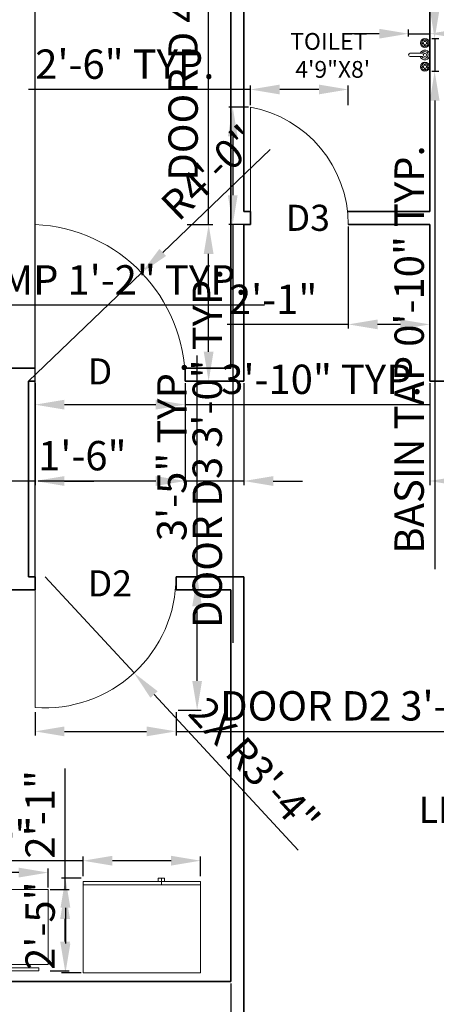
# Model space of a CAD drawing. Units: inches. Extents: x 2396 to 4051, y 1419 to 2191.
# Tile 3 of 7: x 2642 to 2770, y 1726 to 2028. Entities that reach past the tile are written whole.
import ezdxf

# ---------------------------------------------------------------- set-up
doc = ezdxf.new("R2010")
doc.units = ezdxf.units.IN
doc.layers.add('A-ANNO-TEXT', color=114, linetype='Continuous', lineweight=18, true_color=0x139b48)
for name, color, linetype, lineweight in [('A-AREA-IDEN', 6, 'Continuous', 18), ('A-DOOR', 4, 'Continuous', 18), ('A-EQPM', 8, 'Continuous', 18), ('A-FLOR-CASE', 9, 'Continuous', 18), ('A-FLOR-FIXT', 9, 'Continuous', 18), ('A-WALL', 7, 'Continuous', 35), ('S-ANNO-DIMS', 2, 'Continuous', 18)]:
    doc.layers.add(name, color=color, linetype=linetype, lineweight=lineweight)
doc.styles.get("Standard").update_dxf_attribs({"font": 'arial.ttf'})
doc.dimstyles.new('ISO-25', dxfattribs={"dimtxt": 9, "dimasz": 9, "dimexe": 1.25, "dimexo": 0.625, "dimgap": 2, "dimtad": 1, "dimdec": 1, "dimlunit": 4, "dimtxsty": 'Standard', "dimcen": 2.5, "dimadec": 0, "dimazin": 0, "dimtfac": 1, "dimtdec": 1, "dimtmove": 0, "dimatfit": 3, "dimfxl": 1, "dimarcsym": 0})

# ---------------------------------------------------------------- blocks, each defined once
blk = doc.blocks.new('Refrigerator-2 door - 36 in top')
for p, q in [((0, -26.999999), (36, -26.999999)), ((12, -26.999999), (12, -28.999999)), ((11, -27.999999), (11, -28.999999)), ((11, -28.999999), (13, -28.999999)), ((13, -28.999999), (13, -27.999999))]:
    blk.add_line(p, q)
blk.add_lwpolyline([(0, -27.999999), (0, 0), (36, 0), (36, -27.999999)], close=True)
blk = doc.blocks.new('Wall Cabinet - 18 x 12 in side')
for points in [[(-12, -18), (-12, 0), (0, 0), (0, -18)], [(-13, -16.5), (-13, -1.5), (-12.5, -1.5), (-12.5, -16.5)]]:
    blk.add_lwpolyline(points, close=True)
blk = doc.blocks.new('Faucet - Bathroom top')
for p, q in [((-4.107, 0.125), (-4.375, 0.125)), ((-3.75, 0.4788), (-3.75, 0.75)), ((-3.5, 0.482), (-3.5, 0.75)), ((-3.1461, 0.125), (-2.875, 0.125)), ((3.143, 0.125), (2.875, 0.125)), ((3.5, 0.4788), (3.5, 0.75)), ((3.75, 0.482), (3.75, 0.75)), ((4.1039, 0.125), (4.375, 0.125)), ((-4.1039, -0.125), (-4.375, -0.125)), ((-3.75, -0.4821), (-3.75, -0.75)), ((-3.5, -0.4789), (-3.5, -0.75)), ((-3.143, -0.125), (-2.875, -0.125)), ((-0.5, -0.8639), (-0.5, -4.5)), ((0.5, -4.5), (0.5, -0.8631)), ((3.1461, -0.125), (2.875, -0.125)), ((3.5, -0.4821), (3.5, -0.75)), ((3.75, -0.4789), (3.75, -0.75)), ((4.107, -0.125), (4.375, -0.125))]:
    blk.add_line(p, q)
for centre, radius in [((-3.625, 0), 1.375), ((-4.625, 0), 0.2795), ((-3.625, 0), 0.5), ((-3.625, 1), 0.2795), ((-2.625, 0), 0.2795), ((0, 0), 0.5), ((3.625, 0), 1.375), ((2.625, 0), 0.2795), ((3.625, 0), 0.5), ((3.625, 1), 0.2795), ((4.625, 0), 0.2795), ((-3.625, -1), 0.2795), ((3.625, -1), 0.2795)]:
    blk.add_circle(centre, radius)
for centre, radius, start, end in [((-3.625, 0), 1, 105.2407, 164.2093), ((-3.625, 0), 1, 16.44125, 74.07887), ((0, 0), 1.5, 289.6514, 250.3603), ((0, 0), 1, 300.3431, 239.7554), ((3.625, 0), 1, 106.12, 164.0884), ((3.625, 0), 1, 16.23422, 73.90469), ((-3.625, 0), 1, 196.2342, 253.9047), ((-3.625, 0), 1, 286.12, 344.0884), ((3.625, 0), 1, 196.4413, 254.0789), ((3.625, 0), 1, 285.2407, 344.2093), ((0, -4.5), 0.5, 180, 0)]:
    blk.add_arc(centre, radius, start, end)
blk = doc.blocks.new('DOOR-D-48IN')
blk.add_line((0, 0), (0, 48))
blk.add_arc((-2.04, 0), 48.04, 0, 87.5622)
blk = doc.blocks.new('DOOR-D3-36IN')
blk.add_line((30, 0), (30, 36))
blk.add_arc((36.6, 36), 36.6, 180, 259.6111)
blk = doc.blocks.new('DOOR-D2-40IN')
blk.add_line((0, 40.11), (0, 0.11))
blk.add_arc((3.08, 40.11), 40.12, 265.5948, 0)
blk = doc.blocks.new('*D40')
at = {"layer": 'Defpoints', "color": 0, "transparency": 16777216}
for p in [(2545.21, 1942.76), (2559.21, 1942.76), (2559.21, 1940.66)]:
    blk.add_point(p, dxfattribs=at)
at = {"layer": 'S-ANNO-DIMS', "color": 0, "lineweight": -2, "transparency": 16777216}
for p, q in [((2536.21, 1940.66), (2527.21, 1940.66)), ((2545.21, 1942.13), (2545.21, 1939.41)), ((2545.21, 1940.66), (2559.21, 1940.66)), ((2559.21, 1942.13), (2559.21, 1939.41)), ((2568.21, 1940.66), (2717.35, 1940.66))]:
    blk.add_line(p, q, dxfattribs=at)
at = {"layer": 'S-ANNO-DIMS', "color": 0, "transparency": 16777216}
for points in [[(2536.21, 1942.16), (2536.21, 1939.16), (2545.21, 1940.66)], [(2568.21, 1942.16), (2568.21, 1939.16), (2559.21, 1940.66)]]:
    blk.add_solid(points, dxfattribs=at)
at = {"layer": 'S-ANNO-DIMS', "color": 0, "transparency": 16777216, "insert": (2647.28, 1947.18), "char_height": 9, "attachment_point": 5}
blk.add_mtext('TABLE LAMP 1\'-2" TYP.', dxfattribs=at)
blk = doc.blocks.new('*D50')
at = {"layer": 'Defpoints', "color": 0, "transparency": 16777216}
for p in [(2767.98, 2022.3), (2767.98, 2012.3), (2769.48, 2012.3)]:
    blk.add_point(p, dxfattribs=at)
at = {"layer": 'S-ANNO-DIMS', "color": 0, "lineweight": -2, "transparency": 16777216}
for p, q in [((2769.48, 2031.3), (2769.48, 2040.3)), ((2768.61, 2022.3), (2770.73, 2022.3)), ((2769.48, 2022.3), (2769.48, 2012.3)), ((2768.61, 2012.3), (2770.73, 2012.3)), ((2769.48, 2003.3), (2769.48, 1859.68))]:
    blk.add_line(p, q, dxfattribs=at)
at = {"layer": 'S-ANNO-DIMS', "color": 0, "transparency": 16777216}
for points in [[(2767.98, 2031.3), (2770.98, 2031.3), (2769.48, 2022.3)], [(2767.98, 2003.3), (2770.98, 2003.3), (2769.48, 2012.3)]]:
    blk.add_solid(points, dxfattribs=at)
at = {"layer": 'S-ANNO-DIMS', "color": 0, "transparency": 16777216, "insert": (2762.83, 1926.99), "char_height": 9, "attachment_point": 5, "rotation": 90}
blk.add_mtext('BASIN TAP 0\'-10" TYP.', dxfattribs=at)
blk = doc.blocks.new('*D51')
at = {"layer": 'Defpoints', "color": 0, "transparency": 16777216}
for p in [(2761.48, 2022.3), (2767.98, 2023.8), (2767.98, 2022.3)]:
    blk.add_point(p, dxfattribs=at)
at = {"layer": 'S-ANNO-DIMS', "color": 0, "lineweight": -2, "transparency": 16777216}
for p, q in [((2761.48, 2022.93), (2761.48, 2025.05)), ((2767.98, 2022.93), (2767.98, 2025.05)), ((2752.48, 2023.8), (2743.48, 2023.8)), ((2761.48, 2023.8), (2767.98, 2023.8)), ((2776.98, 2023.8), (2865.81, 2023.8))]:
    blk.add_line(p, q, dxfattribs=at)
at = {"layer": 'S-ANNO-DIMS', "color": 0, "transparency": 16777216}
for points in [[(2752.48, 2025.3), (2752.48, 2022.3), (2761.48, 2023.8)], [(2776.98, 2025.3), (2776.98, 2022.3), (2767.98, 2023.8)]]:
    blk.add_solid(points, dxfattribs=at)
at = {"layer": 'S-ANNO-DIMS', "color": 0, "transparency": 16777216, "insert": (2825.9, 2030.45), "char_height": 9, "attachment_point": 5}
blk.add_mtext('0\'-6 1/2" TYP.', dxfattribs=at)
blk = doc.blocks.new('*D56')
at = {"layer": 'Defpoints', "color": 0, "transparency": 16777216}
for p in [(2692.98, 1965.3), (2700.18, 1965.3), (2692.98, 1917.3)]:
    blk.add_point(p, dxfattribs=at)
at = {"layer": 'S-ANNO-DIMS', "color": 0, "lineweight": -2, "transparency": 16777216}
for p, q in [((2700.18, 1965.3), (2700.18, 2086.5)), ((2693.61, 1965.3), (2701.43, 1965.3)), ((2700.18, 1926.3), (2700.18, 1956.3)), ((2693.61, 1917.3), (2701.43, 1917.3))]:
    blk.add_line(p, q, dxfattribs=at)
at = {"layer": 'S-ANNO-DIMS', "color": 0, "transparency": 16777216}
for points in [[(2698.68, 1956.3), (2701.68, 1956.3), (2700.18, 1965.3)], [(2698.68, 1926.3), (2701.68, 1926.3), (2700.18, 1917.3)]]:
    blk.add_solid(points, dxfattribs=at)
at = {"layer": 'S-ANNO-DIMS', "color": 0, "transparency": 16777216, "insert": (2693.53, 2030.4), "char_height": 9, "attachment_point": 5, "rotation": 90}
blk.add_mtext('DOOR D 4\'-0" TYP.', dxfattribs=at)
blk = doc.blocks.new('*D57')
at = {"layer": 'Defpoints', "color": 0, "transparency": 16777216}
for p in [(2646.98, 1917.3), (2692.98, 1917.3), (2692.98, 1910.1)]:
    blk.add_point(p, dxfattribs=at)
at = {"layer": 'S-ANNO-DIMS', "color": 0, "lineweight": -2, "transparency": 16777216}
for p, q in [((2646.98, 1916.68), (2646.98, 1908.85)), ((2692.98, 1916.68), (2692.98, 1908.85)), ((2655.98, 1910.1), (2683.98, 1910.1)), ((2692.98, 1910.1), (2767.83, 1910.1))]:
    blk.add_line(p, q, dxfattribs=at)
at = {"layer": 'S-ANNO-DIMS', "color": 0, "transparency": 16777216}
for points in [[(2655.98, 1911.6), (2655.98, 1908.6), (2646.98, 1910.1)], [(2683.98, 1911.6), (2683.98, 1908.6), (2692.98, 1910.1)]]:
    blk.add_solid(points, dxfattribs=at)
at = {"layer": 'S-ANNO-DIMS', "color": 0, "transparency": 16777216, "insert": (2734.91, 1916.7), "char_height": 9, "attachment_point": 5}
blk.add_mtext('3\'-10" TYP.', dxfattribs=at)
blk = doc.blocks.new('*D58')
at = {"layer": 'Defpoints', "color": 0, "transparency": 16777216}
for p in [(2712.98, 2001.3), (2707.58, 1965.3), (2712.98, 1965.3)]:
    blk.add_point(p, dxfattribs=at)
at = {"layer": 'S-ANNO-DIMS', "color": 0, "lineweight": -2, "transparency": 16777216}
for p, q in [((2712.36, 2001.3), (2706.33, 2001.3)), ((2707.58, 1992.3), (2707.58, 1974.3)), ((2712.36, 1965.3), (2706.33, 1965.3)), ((2707.58, 1965.3), (2707.58, 1837.11))]:
    blk.add_line(p, q, dxfattribs=at)
at = {"layer": 'S-ANNO-DIMS', "color": 0, "transparency": 16777216}
for points in [[(2706.08, 1992.3), (2709.08, 1992.3), (2707.58, 2001.3)], [(2706.08, 1974.3), (2709.08, 1974.3), (2707.58, 1965.3)]]:
    blk.add_solid(points, dxfattribs=at)
at = {"layer": 'S-ANNO-DIMS', "color": 0, "transparency": 16777216, "insert": (2700.92, 1896.71), "char_height": 9, "attachment_point": 5, "rotation": 90}
blk.add_mtext('DOOR D3 3\'-0" TYP.', dxfattribs=at)
blk = doc.blocks.new('*D59')
at = {"layer": 'Defpoints', "color": 0, "transparency": 16777216}
for p in [(2712.98, 2006.7), (2712.98, 2001.3), (2742.98, 2001.3)]:
    blk.add_point(p, dxfattribs=at)
at = {"layer": 'S-ANNO-DIMS', "color": 0, "lineweight": -2, "transparency": 16777216}
for p, q in [((2712.98, 2001.93), (2712.98, 2007.95)), ((2742.98, 2001.93), (2742.98, 2007.95)), ((2712.98, 2006.7), (2644.97, 2006.7)), ((2733.98, 2006.7), (2721.98, 2006.7))]:
    blk.add_line(p, q, dxfattribs=at)
at = {"layer": 'S-ANNO-DIMS', "color": 0, "transparency": 16777216}
for points in [[(2721.98, 2008.2), (2721.98, 2005.2), (2712.98, 2006.7)], [(2733.98, 2008.2), (2733.98, 2005.2), (2742.98, 2006.7)]]:
    blk.add_solid(points, dxfattribs=at)
at = {"layer": 'S-ANNO-DIMS', "color": 0, "transparency": 16777216, "insert": (2674.48, 2013.3), "char_height": 9, "attachment_point": 5}
blk.add_mtext('2\'-6" TYP.', dxfattribs=at)
blk = doc.blocks.new('*D60')
at = {"layer": 'Defpoints', "color": 0, "transparency": 16777216}
for p in [(2646.98, 1816.44), (2690.18, 1816.44), (2690.18, 1809.96)]:
    blk.add_point(p, dxfattribs=at)
at = {"layer": 'S-ANNO-DIMS', "color": 0, "lineweight": -2, "transparency": 16777216}
for p, q in [((2646.98, 1815.82), (2646.98, 1808.71)), ((2690.18, 1815.82), (2690.18, 1808.71)), ((2655.98, 1809.96), (2681.18, 1809.96)), ((2690.18, 1809.96), (2818.37, 1809.96))]:
    blk.add_line(p, q, dxfattribs=at)
at = {"layer": 'S-ANNO-DIMS', "color": 0, "transparency": 16777216}
for points in [[(2655.98, 1811.46), (2655.98, 1808.46), (2646.98, 1809.96)], [(2681.18, 1811.46), (2681.18, 1808.46), (2690.18, 1809.96)]]:
    blk.add_solid(points, dxfattribs=at)
at = {"layer": 'S-ANNO-DIMS', "color": 0, "transparency": 16777216, "insert": (2758.78, 1816.62), "char_height": 9, "attachment_point": 5}
blk.add_mtext('DOOR D2 3\'-7" TYP.', dxfattribs=at)
blk = doc.blocks.new('*D61')
at = {"layer": 'Defpoints', "color": 0, "transparency": 16777216}
for p in [(2690.18, 1857.3), (2696.66, 1857.3), (2690.18, 1816.44)]:
    blk.add_point(p, dxfattribs=at)
at = {"layer": 'S-ANNO-DIMS', "color": 0, "lineweight": -2, "transparency": 16777216}
for p, q in [((2696.66, 1857.3), (2696.66, 1925.15)), ((2690.81, 1857.3), (2697.91, 1857.3)), ((2696.66, 1825.44), (2696.66, 1848.3)), ((2690.81, 1816.44), (2697.91, 1816.44))]:
    blk.add_line(p, q, dxfattribs=at)
at = {"layer": 'S-ANNO-DIMS', "color": 0, "transparency": 16777216}
for points in [[(2695.16, 1848.3), (2698.16, 1848.3), (2696.66, 1857.3)], [(2695.16, 1825.44), (2698.16, 1825.44), (2696.66, 1816.44)]]:
    blk.add_solid(points, dxfattribs=at)
at = {"layer": 'S-ANNO-DIMS', "color": 0, "transparency": 16777216, "insert": (2690.07, 1895.73), "char_height": 9, "attachment_point": 5, "rotation": 90}
blk.add_mtext('3\'-5" TYP.', dxfattribs=at)
blk = doc.blocks.new('*D66')
at = {"layer": 'Defpoints', "color": 0, "transparency": 16777216}
for p in [(2661.68, 1770.32), (2661.68, 1764.92), (2697.68, 1764.92)]:
    blk.add_point(p, dxfattribs=at)
at = {"layer": 'S-ANNO-DIMS', "color": 0, "lineweight": -2, "transparency": 16777216}
for p, q in [((2661.68, 1765.55), (2661.68, 1771.57)), ((2697.68, 1765.55), (2697.68, 1771.57)), ((2661.68, 1770.32), (2521.84, 1770.32)), ((2688.68, 1770.32), (2670.68, 1770.32))]:
    blk.add_line(p, q, dxfattribs=at)
at = {"layer": 'S-ANNO-DIMS', "color": 0, "transparency": 16777216}
for points in [[(2670.68, 1771.82), (2670.68, 1768.82), (2661.68, 1770.32)], [(2688.68, 1771.82), (2688.68, 1768.82), (2697.68, 1770.32)]]:
    blk.add_solid(points, dxfattribs=at)
at = {"layer": 'S-ANNO-DIMS', "color": 0, "transparency": 16777216, "insert": (2587.26, 1776.98), "char_height": 9, "attachment_point": 5}
blk.add_mtext('REFRIGERATOR 3\'-0"', dxfattribs=at)
blk = doc.blocks.new('*D67')
at = {"layer": 'Defpoints', "color": 0, "transparency": 16777216}
for p in [(2661.68, 1764.92), (2656.28, 1735.92), (2661.68, 1735.92)]:
    blk.add_point(p, dxfattribs=at)
at = {"layer": 'S-ANNO-DIMS', "color": 0, "lineweight": -2, "transparency": 16777216}
for p, q in [((2661.06, 1764.92), (2655.03, 1764.92)), ((2656.28, 1755.92), (2656.28, 1744.92)), ((2661.06, 1735.92), (2655.03, 1735.92))]:
    blk.add_line(p, q, dxfattribs=at)
at = {"layer": 'S-ANNO-DIMS', "color": 0, "transparency": 16777216}
for points in [[(2654.78, 1755.92), (2657.78, 1755.92), (2656.28, 1764.92)], [(2654.78, 1744.92), (2657.78, 1744.92), (2656.28, 1735.92)]]:
    blk.add_solid(points, dxfattribs=at)
at = {"layer": 'S-ANNO-DIMS', "color": 0, "transparency": 16777216, "insert": (2649.69, 1750.42), "char_height": 9, "attachment_point": 5, "rotation": 90}
blk.add_mtext('2\'-5"', dxfattribs=at)
blk = doc.blocks.new('*D68')
at = {"layer": 'Defpoints', "color": 0, "transparency": 16777216}
for p in [(2616.45, 1766.68), (2616.45, 1761.5), (2650.99, 1761.5)]:
    blk.add_point(p, dxfattribs=at)
at = {"layer": 'S-ANNO-DIMS', "color": 0, "lineweight": -2, "transparency": 16777216}
for p, q in [((2616.45, 1766.68), (2493.68, 1766.68)), ((2616.45, 1762.12), (2616.45, 1767.93)), ((2641.99, 1766.68), (2625.45, 1766.68)), ((2650.99, 1762.12), (2650.99, 1767.93))]:
    blk.add_line(p, q, dxfattribs=at)
at = {"layer": 'S-ANNO-DIMS', "color": 0, "transparency": 16777216}
for points in [[(2625.45, 1768.18), (2625.45, 1765.18), (2616.45, 1766.68)], [(2641.99, 1768.18), (2641.99, 1765.18), (2650.99, 1766.68)]]:
    blk.add_solid(points, dxfattribs=at)
at = {"layer": 'S-ANNO-DIMS', "color": 0, "transparency": 16777216, "insert": (2550.56, 1773.33), "char_height": 9, "attachment_point": 5}
blk.add_mtext('CABINET 2\'-10 1/2"', dxfattribs=at)
blk = doc.blocks.new('*D69')
at = {"layer": 'Defpoints', "color": 0, "transparency": 16777216}
for p in [(2650.99, 1761.5), (2656.17, 1761.5), (2650.99, 1736.54)]:
    blk.add_point(p, dxfattribs=at)
at = {"layer": 'S-ANNO-DIMS', "color": 0, "lineweight": -2, "transparency": 16777216}
for p, q in [((2656.17, 1761.5), (2656.17, 1798.57)), ((2651.62, 1761.5), (2657.42, 1761.5)), ((2656.17, 1745.54), (2656.17, 1752.5)), ((2651.62, 1736.54), (2657.42, 1736.54))]:
    blk.add_line(p, q, dxfattribs=at)
at = {"layer": 'S-ANNO-DIMS', "color": 0, "transparency": 16777216}
for points in [[(2654.67, 1752.5), (2657.67, 1752.5), (2656.17, 1761.5)], [(2654.67, 1745.54), (2657.67, 1745.54), (2656.17, 1736.54)]]:
    blk.add_solid(points, dxfattribs=at)
at = {"layer": 'S-ANNO-DIMS', "color": 0, "transparency": 16777216, "insert": (2649.66, 1784.53), "char_height": 9, "attachment_point": 5, "rotation": 90}
blk.add_mtext('2\'-1"', dxfattribs=at)
blk = doc.blocks.new('*D77')
at = {"layer": 'Defpoints', "color": 0, "transparency": 16777216}
for p in [(2529.98, 2074.3), (2499.38, 1534.3), (2774.98, 1534.3)]:
    blk.add_point(p, dxfattribs=at)
at = {"layer": 'S-ANNO-DIMS', "color": 0, "lineweight": -2, "transparency": 16777216}
for p, q in [((2529.36, 2074.3), (2498.13, 2074.3)), ((2499.38, 2065.3), (2499.38, 1543.3)), ((2774.36, 1534.3), (2498.13, 1534.3))]:
    blk.add_line(p, q, dxfattribs=at)
at = {"layer": 'S-ANNO-DIMS', "color": 0, "transparency": 16777216}
for points in [[(2497.88, 2065.3), (2500.88, 2065.3), (2499.38, 2074.3)], [(2497.88, 1543.3), (2500.88, 1543.3), (2499.38, 1534.3)]]:
    blk.add_solid(points, dxfattribs=at)
at = {"layer": 'S-ANNO-DIMS', "color": 0, "transparency": 16777216, "insert": (2492.79, 1804.3), "char_height": 9, "attachment_point": 5, "rotation": 90}
blk.add_mtext('45\'-0"', dxfattribs=at)
blk = doc.blocks.new('*D78')
at = {"layer": 'Defpoints', "color": 0, "transparency": 16777216}
for p in [(2538.98, 1733.3), (2706.98, 1733.3), (2706.98, 1503.7)]:
    blk.add_point(p, dxfattribs=at)
at = {"layer": 'S-ANNO-DIMS', "color": 0, "lineweight": -2, "transparency": 16777216}
for p, q in [((2538.98, 1732.68), (2538.98, 1502.45)), ((2706.98, 1732.68), (2706.98, 1502.45)), ((2547.98, 1503.7), (2697.98, 1503.7))]:
    blk.add_line(p, q, dxfattribs=at)
at = {"layer": 'S-ANNO-DIMS', "color": 0, "transparency": 16777216}
for points in [[(2547.98, 1505.2), (2547.98, 1502.2), (2538.98, 1503.7)], [(2697.98, 1505.2), (2697.98, 1502.2), (2706.98, 1503.7)]]:
    blk.add_solid(points, dxfattribs=at)
at = {"layer": 'S-ANNO-DIMS', "color": 0, "transparency": 16777216, "insert": (2622.98, 1510.3), "char_height": 9, "attachment_point": 5}
blk.add_mtext('14\'-0"', dxfattribs=at)
blk = doc.blocks.new('*D94')
at = {"layer": 'Defpoints', "color": 0, "transparency": 16777216}
for p in [(2767.98, 1917.3), (2846.98, 1917.3), (2767.98, 1886.7)]:
    blk.add_point(p, dxfattribs=at)
at = {"layer": 'S-ANNO-DIMS', "color": 0, "lineweight": -2, "transparency": 16777216}
for p, q in [((2767.98, 1916.68), (2767.98, 1885.45)), ((2846.98, 1916.68), (2846.98, 1885.45)), ((2837.98, 1886.7), (2776.98, 1886.7))]:
    blk.add_line(p, q, dxfattribs=at)
at = {"layer": 'S-ANNO-DIMS', "color": 0, "transparency": 16777216}
for points in [[(2776.98, 1888.2), (2776.98, 1885.2), (2767.98, 1886.7)], [(2837.98, 1888.2), (2837.98, 1885.2), (2846.98, 1886.7)]]:
    blk.add_solid(points, dxfattribs=at)
at = {"layer": 'S-ANNO-DIMS', "color": 0, "transparency": 16777216, "insert": (2807.48, 1893.3), "char_height": 9, "attachment_point": 5}
blk.add_mtext('6\'-7"', dxfattribs=at)
blk = doc.blocks.new('*D95')
at = {"layer": 'Defpoints', "color": 0, "transparency": 16777216}
for p in [(2646.98, 2154.77), (2538.98, 1853.3), (2646.98, 1853.3)]:
    blk.add_point(p, dxfattribs=at)
at = {"layer": 'S-ANNO-DIMS', "color": 0, "lineweight": -2, "transparency": 16777216}
for p, q in [((2538.98, 1853.93), (2538.98, 2156.02)), ((2547.98, 2154.77), (2637.98, 2154.77)), ((2646.98, 1853.93), (2646.98, 2156.02))]:
    blk.add_line(p, q, dxfattribs=at)
at = {"layer": 'S-ANNO-DIMS', "color": 0, "transparency": 16777216}
for points in [[(2547.98, 2156.27), (2547.98, 2153.27), (2538.98, 2154.77)], [(2637.98, 2156.27), (2637.98, 2153.27), (2646.98, 2154.77)]]:
    blk.add_solid(points, dxfattribs=at)
at = {"layer": 'S-ANNO-DIMS', "color": 0, "transparency": 16777216, "insert": (2592.98, 2161.37), "char_height": 9, "attachment_point": 5}
blk.add_mtext('9\'-0"', dxfattribs=at)
blk = doc.blocks.new('*D97')
at = {"layer": 'Defpoints', "color": 0, "transparency": 16777216}
for p in [(2692.98, 1917.3), (2710.98, 1917.3), (2692.98, 1886.7)]:
    blk.add_point(p, dxfattribs=at)
at = {"layer": 'S-ANNO-DIMS', "color": 0, "lineweight": -2, "transparency": 16777216}
for p, q in [((2692.98, 1916.68), (2692.98, 1885.45)), ((2710.98, 1916.68), (2710.98, 1885.45)), ((2683.98, 1886.7), (2647.91, 1886.7)), ((2710.98, 1886.7), (2692.98, 1886.7)), ((2719.98, 1886.7), (2728.98, 1886.7))]:
    blk.add_line(p, q, dxfattribs=at)
at = {"layer": 'S-ANNO-DIMS', "color": 0, "transparency": 16777216}
for points in [[(2683.98, 1888.2), (2683.98, 1885.2), (2692.98, 1886.7)], [(2719.98, 1888.2), (2719.98, 1885.2), (2710.98, 1886.7)]]:
    blk.add_solid(points, dxfattribs=at)
at = {"layer": 'S-ANNO-DIMS', "color": 0, "transparency": 16777216, "insert": (2661.45, 1893.3), "char_height": 9, "attachment_point": 5}
blk.add_mtext('1\'-6"', dxfattribs=at)
blk = doc.blocks.new('*D98')
at = {"layer": 'Defpoints', "color": 0, "transparency": 16777216}
for p in [(2629.98, 1917.3), (2646.98, 1917.3), (2629.98, 1886.7)]:
    blk.add_point(p, dxfattribs=at)
at = {"layer": 'S-ANNO-DIMS', "color": 0, "lineweight": -2, "transparency": 16777216}
for p, q in [((2629.98, 1916.68), (2629.98, 1885.45)), ((2646.98, 1916.68), (2646.98, 1885.45)), ((2620.98, 1886.7), (2584.91, 1886.7)), ((2646.98, 1886.7), (2629.98, 1886.7)), ((2655.98, 1886.7), (2664.98, 1886.7))]:
    blk.add_line(p, q, dxfattribs=at)
at = {"layer": 'S-ANNO-DIMS', "color": 0, "transparency": 16777216}
for points in [[(2620.98, 1888.2), (2620.98, 1885.2), (2629.98, 1886.7)], [(2655.98, 1888.2), (2655.98, 1885.2), (2646.98, 1886.7)]]:
    blk.add_solid(points, dxfattribs=at)
at = {"layer": 'S-ANNO-DIMS', "color": 0, "transparency": 16777216, "insert": (2598.45, 1893.3), "char_height": 9, "attachment_point": 5}
blk.add_mtext('1\'-5"', dxfattribs=at)
blk = doc.blocks.new('*D99')
at = {"layer": 'Defpoints', "color": 0, "transparency": 16777216}
for p in [(2742.98, 1965.3), (2767.98, 1965.3), (2742.98, 1934.7)]:
    blk.add_point(p, dxfattribs=at)
at = {"layer": 'S-ANNO-DIMS', "color": 0, "lineweight": -2, "transparency": 16777216}
for p, q in [((2742.98, 1964.68), (2742.98, 1933.45)), ((2767.98, 1964.68), (2767.98, 1933.45)), ((2742.98, 1934.7), (2705.91, 1934.7)), ((2758.98, 1934.7), (2751.98, 1934.7))]:
    blk.add_line(p, q, dxfattribs=at)
at = {"layer": 'S-ANNO-DIMS', "color": 0, "transparency": 16777216}
for points in [[(2751.98, 1936.2), (2751.98, 1933.2), (2742.98, 1934.7)], [(2758.98, 1936.2), (2758.98, 1933.2), (2767.98, 1934.7)]]:
    blk.add_solid(points, dxfattribs=at)
at = {"layer": 'S-ANNO-DIMS', "color": 0, "transparency": 16777216, "insert": (2719.95, 1941.22), "char_height": 9, "attachment_point": 5}
blk.add_mtext('2\'-1"', dxfattribs=at)
blk = doc.blocks.new('*D113')
at = {"layer": 'Defpoints', "color": 0, "transparency": 16777216}
for p in [(2679.63, 1950.54), (2644.94, 1917.3)]:
    blk.add_point(p, dxfattribs=at)
at = {"layer": 'S-ANNO-DIMS', "color": 0, "lineweight": -2, "transparency": 16777216}
for p, q in [((2719, 1988.28), (2686.13, 1956.77)), ((2644.94, 1917.3), (2679.63, 1950.54))]:
    blk.add_line(p, q, dxfattribs=at)
at = {"layer": 'S-ANNO-DIMS', "color": 0, "transparency": 16777216}
blk.add_solid([(2685.09, 1957.85), (2687.16, 1955.69), (2679.63, 1950.54)], dxfattribs=at)
at = {"layer": 'S-ANNO-DIMS', "color": 0, "transparency": 16777216, "insert": (2701.25, 1980.4), "char_height": 9, "attachment_point": 5, "rotation": 43.7812}
blk.add_mtext('R4\'-0"', dxfattribs=at)
blk = doc.blocks.new('*D114')
at = {"layer": 'Defpoints', "color": 0, "transparency": 16777216}
for p in [(2650.07, 1857.3), (2677.32, 1827.86)]:
    blk.add_point(p, dxfattribs=at)
at = {"layer": 'S-ANNO-DIMS', "color": 0, "lineweight": -2, "transparency": 16777216}
for p, q in [((2650.07, 1857.3), (2677.32, 1827.86)), ((2727.62, 1773.54), (2683.44, 1821.26))]:
    blk.add_line(p, q, dxfattribs=at)
at = {"layer": 'S-ANNO-DIMS', "color": 0, "transparency": 16777216}
blk.add_solid([(2684.54, 1822.28), (2682.34, 1820.24), (2677.32, 1827.86)], dxfattribs=at)
at = {"layer": 'S-ANNO-DIMS', "color": 0, "transparency": 16777216, "insert": (2713.43, 1798.58), "char_height": 9, "attachment_point": 5, "rotation": 312.7969}
blk.add_mtext('2X R3\'-4"', dxfattribs=at)

msp = doc.modelspace()

# ---------------------------------------------------------------- linework, layer by layer
at = {"layer": 'A-WALL'}
for p, q in [((2706.98, 2065.3), (2706.98, 1921.3)), ((2710.98, 2065.3), (2710.98, 1969.3)), ((2767.98, 2065.3), (2767.98, 1969.3)), ((2710.98, 1969.3), (2712.98, 1969.3)), ((2712.98, 1969.3), (2712.98, 1965.3)), ((2742.76, 1969.3), (2767.98, 1969.3)), ((2710.98, 1965.3), (2712.98, 1965.3)), ((2710.98, 1965.3), (2710.98, 1917.3)), ((2742.98, 1965.3), (2767.98, 1965.3)), ((2767.98, 1965.3), (2767.98, 1917.3)), ((2646.98, 1921.3), (2629.98, 1921.3)), ((2706.98, 1921.3), (2692.98, 1921.3)), ((2692.98, 1917.3), (2692.98, 1921.3)), ((2644.98, 1857.3), (2644.98, 1917.3)), ((2646.98, 1917.3), (2644.98, 1917.3)), ((2710.98, 1917.3), (2692.98, 1917.3)), ((2846.98, 1917.3), (2767.98, 1917.3)), ((2646.98, 1857.3), (2644.98, 1857.3)), ((2646.98, 1853.3), (2646.98, 1857.3)), ((2710.98, 1857.3), (2690.18, 1857.3)), ((2690.18, 1853.3), (2690.18, 1857.3)), ((2710.98, 1857.3), (2710.98, 1632.3)), ((2644.98, 1853.3), (2538.98, 1853.3)), ((2646.98, 1853.3), (2644.98, 1853.3)), ((2706.98, 1853.3), (2690.18, 1853.3)), ((2706.98, 1853.3), (2706.98, 1733.3)), ((2706.98, 1733.3), (2538.98, 1733.3))]:
    msp.add_line(p, q, dxfattribs=at)

# ---------------------------------------------------------------- block references
at = {"layer": 'A-DOOR', "rotation": 180}
msp.add_blockref('DOOR-D3-36IN', (2742.98, 2001.3), dxfattribs=at)
at = {"layer": 'A-DOOR'}
for name, p in [('DOOR-D-48IN', (2646.98, 1917.3)), ('DOOR-D2-40IN', (2646.98, 1817.19))]:
    msp.add_blockref(name, p, dxfattribs=at)
at = {"layer": 'A-EQPM', "rotation": 180}
msp.add_blockref('Refrigerator-2 door - 36 in top', (2697.68, 1735.92), dxfattribs=at)
at = {"layer": 'A-FLOR-CASE', "xscale": 1.91927912988188, "yscale": 1.91927912988188, "zscale": 1.91927912988188, "rotation": 90}
msp.add_blockref('Wall Cabinet - 18 x 12 in side', (2616.45, 1761.5), dxfattribs=at)
at = {"layer": 'A-FLOR-FIXT', "rotation": 270}
msp.add_blockref('Faucet - Bathroom top', (2766.48, 2017.3), dxfattribs=at)

# ---------------------------------------------------------------- texts
at = {"layer": 'A-ANNO-TEXT', "char_height": 8, "attachment_point": 1}
for s, insert in [('{D3}', (2723.8, 1971.37)), ('{D}', (2663.12, 1924.28)), ('{D2}', (2663.12, 1859.32))]:
    msp.add_mtext_dynamic_manual_height_columns(s, width=139.3028, gutter_width=12.5, heights=[0], dxfattribs=dict(at, insert=insert))
at = {"layer": 'A-AREA-IDEN', "attachment_point": 1}
for s, width, gutter_width, insert, char_height in [('   TOILET\\P    4\'9"X8\'', 89.5376, 8.03, (2720.48, 2024.01), 5.142), ("   LIVING ROOM\\P        15'X23'", 139.3028, 12.5, (2757.3, 1789.91), 8)]:
    msp.add_mtext_dynamic_manual_height_columns(s, width=width, gutter_width=gutter_width, heights=[0], dxfattribs=dict(at, insert=insert, char_height=char_height))

# ---------------------------------------------------------------- dimensions: what is measured, and where the dimension line sits
at = {"layer": 'S-ANNO-DIMS'}
for base, p1, p2, picture, middle in [((2646.98, 2154.77), (2538.98, 1853.3), (2646.98, 1853.3), '*D95', (2592.98, 2161.37)), ((2706.98, 1503.7), (2538.98, 1733.3), (2706.98, 1733.3), '*D78', (2622.98, 1510.3))]:
    dim = msp.add_linear_dim(base=base, p1=p1, p2=p2, dimstyle='ISO-25', override={"dimdec": 1, "dimlfac": 1, "dimrnd": 0, "dimzin": 1, "dimdsep": 46, "dimlunit": 4, "dimfrac": 2}, dxfattribs=at)
    dim.commit()
    dim.dimension.update_dxf_attribs({"geometry": picture, "text_midpoint": middle})
for base, p1, p2, angle, text, picture, middle in [((2700.18, 1965.3), (2692.98, 1917.3), (2692.98, 1965.3), 90, 'DOOR D <> TYP.', '*D56', (2693.53, 2030.4)), ((2769.48, 2012.3), (2767.98, 2022.3), (2767.98, 2012.3), 270, 'BASIN TAP <> TYP.', '*D50', (2762.83, 1926.99)), ((2712.98, 2006.7), (2742.98, 2001.3), (2712.98, 2001.3), 180, '<> TYP.', '*D59', (2674.48, 2013.3)), ((2707.58, 1965.3), (2712.98, 2001.3), (2712.98, 1965.3), 270, 'DOOR D3 <> TYP.', '*D58', (2700.92, 1896.71)), ((2696.66, 1857.3), (2690.18, 1816.44), (2690.18, 1857.3), 90, '<> TYP.', '*D61', (2690.07, 1895.73)), ((2616.45, 1766.68), (2650.99, 1761.5), (2616.45, 1761.5), 180, 'CABINET <>', '*D68', (2550.56, 1773.33)), ((2661.68, 1770.32), (2697.68, 1764.92), (2661.68, 1764.92), 180, 'REFRIGERATOR <>', '*D66', (2587.26, 1776.98))]:
    dim = msp.add_linear_dim(base=base, p1=p1, p2=p2, angle=angle, text=text, dimstyle='ISO-25', override={"dimdec": 1, "dimlfac": 1, "dimrnd": 0, "dimzin": 1, "dimdsep": 46, "dimlunit": 4, "dimfrac": 2}, dxfattribs=at)
    dim.commit()
    dim.dimension.update_dxf_attribs({"geometry": picture, "text_midpoint": middle})
for base, p1, p2, angle, picture, middle in [((2499.38, 1534.3), (2529.98, 2074.3), (2774.98, 1534.3), 90, '*D77', (2492.79, 1804.3)), ((2742.98, 1934.7), (2767.98, 1965.3), (2742.98, 1965.3), 180, '*D99', (2719.95, 1941.22)), ((2629.98, 1886.7), (2646.98, 1917.3), (2629.98, 1917.3), 180, '*D98', (2598.45, 1893.3)), ((2692.98, 1886.7), (2710.98, 1917.3), (2692.98, 1917.3), 180, '*D97', (2661.45, 1893.3)), ((2767.98, 1886.7), (2846.98, 1917.3), (2767.98, 1917.3), 180, '*D94', (2807.48, 1893.3)), ((2656.17, 1761.5), (2650.99, 1736.54), (2650.99, 1761.5), 90, '*D69', (2649.66, 1784.53)), ((2656.28, 1735.92), (2661.68, 1764.92), (2661.68, 1735.92), 270, '*D67', (2649.69, 1750.42))]:
    dim = msp.add_linear_dim(base=base, p1=p1, p2=p2, angle=angle, dimstyle='ISO-25', override={"dimdec": 1, "dimlfac": 1, "dimrnd": 0, "dimzin": 1, "dimdsep": 46, "dimlunit": 4, "dimfrac": 2}, dxfattribs=at)
    dim.commit()
    dim.dimension.update_dxf_attribs({"geometry": picture, "text_midpoint": middle})
for base, p1, p2, text, picture, middle in [((2767.98, 2023.8), (2761.48, 2022.3), (2767.98, 2022.3), '<> TYP.', '*D51', (2825.9, 2030.45)), ((2559.21, 1940.66), (2545.21, 1942.76), (2559.21, 1942.76), 'TABLE LAMP <> TYP.', '*D40', (2647.28, 1947.18)), ((2692.98, 1910.1), (2646.98, 1917.3), (2692.98, 1917.3), '<> TYP.', '*D57', (2734.91, 1916.7)), ((2690.18, 1809.96), (2646.98, 1816.44), (2690.18, 1816.44), 'DOOR D2 <> TYP.', '*D60', (2758.78, 1816.62))]:
    dim = msp.add_linear_dim(base=base, p1=p1, p2=p2, text=text, dimstyle='ISO-25', override={"dimdec": 1, "dimlfac": 1, "dimrnd": 0, "dimzin": 1, "dimdsep": 46, "dimlunit": 4, "dimfrac": 2}, dxfattribs=at)
    dim.commit()
    dim.dimension.update_dxf_attribs({"geometry": picture, "text_midpoint": middle})
dim = msp.add_radius_dim(center=(2644.94, 1917.3), mpoint=(2679.63, 1950.54), dimstyle='ISO-25', override={"dimdec": 1, "dimlfac": 1, "dimrnd": 0, "dimzin": 1, "dimdsep": 46, "dimlunit": 4, "dimfrac": 2}, dxfattribs=at)
dim.commit()
dim.dimension.update_dxf_attribs({"geometry": '*D113', "text_midpoint": (2701.25, 1980.4)})
dim = msp.add_radius_dim(center=(2650.07, 1857.3), mpoint=(2677.32, 1827.86), text='2X <>', dimstyle='ISO-25', override={"dimdec": 1, "dimlfac": 1, "dimrnd": 0, "dimzin": 1, "dimdsep": 46, "dimlunit": 4, "dimfrac": 2}, dxfattribs=at)
dim.commit()
dim.dimension.update_dxf_attribs({"geometry": '*D114', "text_midpoint": (2713.43, 1798.58)})

doc.saveas('drawing.dxf')
